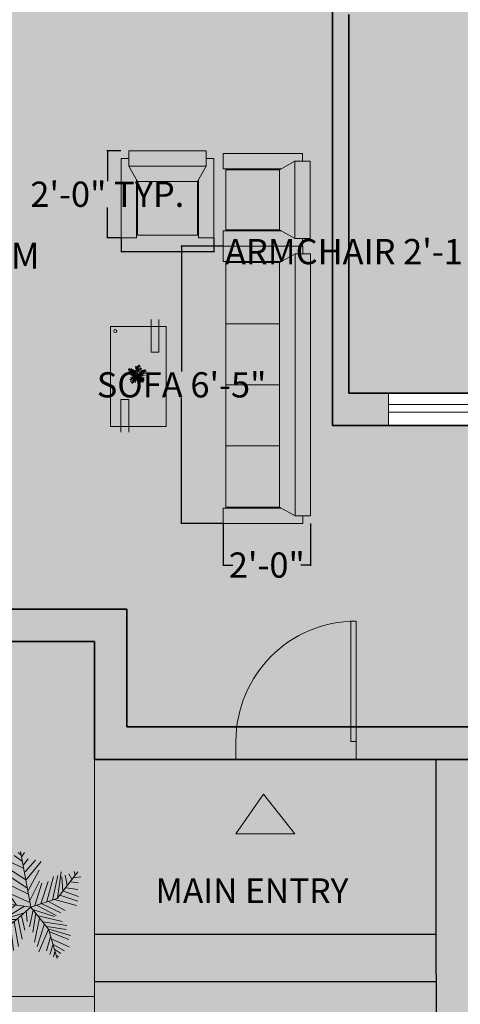
# Model space of a CAD drawing. Units: inches. Extents: x 1316 to 1777, y 813 to 1650.
# Tile 3 of 22: x 1481 to 1603, y 963 to 1237. Entities that reach past the tile are written whole.
import ezdxf

# ---------------------------------------------------------------- set-up
doc = ezdxf.new("R2010")
doc.units = ezdxf.units.IN
doc.header["$MEASUREMENT"] = 0
for name, color, linetype, lineweight in [('A-ANNO-DIMS', 2, 'Continuous', 18), ('A-ANNO-SYMB', 7, 'Continuous', 18), ('A-ANNO-SYMB-PATT', 7, 'Continuous', 13), ('A-AREA-IDEN', 7, 'Continuous', 18), ('A-DOOR', 4, 'Continuous', 18), ('A-DOOR-PATT', 253, 'Continuous', 13), ('A-FLOR-STRS', 7, 'Continuous', 25), ('A-FLOR-STRS-PATT', 252, 'Continuous', 13), ('A-FURN-PATT', 23, 'Continuous', 13), ('A-WALL-PATT', 250, 'Continuous', 13), ('furniture', 23, 'Continuous', 18), ('greenary', 106, 'Continuous', 13), ('L-HRDS', 8, 'Continuous', 18), ('L-HRDS-PATT', 252, 'Continuous', 13), ('L-PLNT-PATT', 74, 'Continuous', 13), ('text', 7, 'Continuous', 18), ('walls', 250, 'Continuous', 35), ('windows', 141, 'Continuous', 18)]:
    doc.layers.add(name, color=color, linetype=linetype, lineweight=lineweight)
doc.layers.add('A-FLOR-PATT', color=254, linetype='Continuous', lineweight=13, true_color=0xfeeab9)
doc.styles.get("Standard").update_dxf_attribs({"font": 'arial.ttf'})
doc.dimstyles.get("Standard").update_dxf_attribs({"dimtxt": 7, "dimasz": 0.18, "dimexe": 0.18, "dimexo": 0.0625, "dimgap": 0.09, "dimtad": 0, "dimtih": 1, "dimtoh": 1, "dimzin": 0, "dimdsep": 46, "dimlunit": 3, "dimtxsty": 'Standard', "dimcen": 0.09, "dimadec": 0, "dimazin": 0, "dimtfac": 1, "dimtofl": 0, "dimtmove": 0, "dimatfit": 3, "dimfxl": 1, "dimtolj": 1, "dimtzin": 0, "dimarcsym": 0})

# ---------------------------------------------------------------- blocks, each defined once
blk = doc.blocks.new('*U15')
for p, q in [((0, 0), (0, -6)), ((40, 0), (40, -6))]:
    blk.add_line(p, q)
blk.add_lwpolyline([(0, 0), (0, 40), (1.75, 40), (1.75, 0)], close=True)
blk.add_arc((0, 0), 40, 0, 90)
blk = doc.blocks.new('FABRIC SOFA 4S')
at = {"layer": 'furniture'}
for p, q in [((3, 54), (34, 54)), ((3, 51), (3, 54)), ((34, 48), (34, 54)), ((0, -51), (0, 51)), ((6, 51), (0, 51)), ((6, -51), (6, 51)), ((12, 47.63), (6, 51)), ((11.14, 48), (34, 48)), ((33, 23.81), (12, 23.81)), ((33, 0), (12, 0)), ((33, -23.81), (12, -23.81)), ((6, -51), (12, -47.63)), ((11.54, -48), (34, -48)), ((34, -48), (34, -54)), ((6, -51), (0, -51)), ((3, -54), (3, -51)), ((3, -54), (34, -54))]:
    blk.add_line(p, q, dxfattribs=at)
blk.add_lwpolyline([(12, -47.63), (12, 47.63), (33, 47.63), (33, -47.63)], close=True, dxfattribs=at)
blk = doc.blocks.new('*U13')
for p, q in [((-8.737, 47.138), (-17.069, 52.711)), ((-10.186, 53.64), (-13.084, 55.962)), ((0, 0), (-10.5, 57)), ((-9.099, 51.782), (-6.563, 55.962)), ((-5.114, 28.097), (-24.676, 40.636)), ((-7.288, 39.707), (-21.778, 46.673)), ((-7.65, 43.423), (-2.578, 49.46)), ((-5.839, 35.992), (4.667, 48.067)), ((-5.114, 27.632), (10.463, 46.673)), ((-3.665, 19.273), (-27.574, 35.527)), ((-2.941, 16.486), (8.652, 37.85)), ((16.259, 5.805), (23.142, 31.348)), ((22.055, 7.198), (27.489, 32.277)), ((27, 9), (48, 36)), ((27.127, 9.056), (31.112, 35.992)), ((31.836, 30.883), (32.561, 16.486)), ((35.096, 32.741), (37.27, 22.524)), ((38.719, 34.134), (41.979, 28.561)), ((43.791, 29.954), (51.036, 30.883)), ((44.153, 36.456), (45.239, 32.741)), ((-31.5, 4.5), (-52.5, 25.5)), ((-48.585, 21.131), (-49.309, 29.026)), ((-43.513, 28.561), (-42.427, 15.558)), ((-38.442, 26.239), (-34.819, 7.663)), ((-35.544, 28.097), (-24.314, 3.947)), ((-14.533, 2.09), (-30.834, 25.31)), ((-24.314, 23.917), (-2.941, 13.7)), ((-1.129, 6.734), (9.014, 26.704)), ((3.942, 1.625), (11.187, 24.381)), ((10.101, 3.483), (17.708, 26.239)), ((40.53, 25.775), (48.862, 24.846)), ((-47.498, 19.737), (-55.83, 18.344)), ((-40.615, 13.7), (-55.105, 10.913)), ((-20.691, 13.7), (-1.129, 4.876)), ((29.662, 12.307), (48.137, 6.269)), ((33.285, 16.486), (48.862, 10.913)), ((36.183, 19.737), (48.137, 17.88)), ((-33.37, 6.269), (-52.207, 5.34)), ((-28.299, 3.483), (-47.86, -5.805)), ((-21.416, 3.018), (-38.079, -8.128)), ((0, 0), (-31.5, 4.5)), ((-15.982, 2.09), (-30.11, -9.521)), ((0, 0), (-22.5, -19.5)), ((-6.563, 1.161), (-21.416, -8.128)), ((0, 0), (27, 9)), ((0, 0), (18, -22.5)), ((6.478, 1.625), (26.04, -8.592)), ((11.187, 3.483), (30.749, -5.805)), ((18.07, 5.805), (35.096, -3.483)), ((24.229, 7.663), (46.688, 1.625)), ((-6.563, -5.805), (-19.967, -9.985)), ((-9.461, -8.592), (-6.201, -23.453)), ((-4.752, -3.483), (-3.665, -14.629)), ((2.493, -3.019), (-1.491, -20.202)), ((1.769, -2.555), (24.229, -9.521)), ((5.029, -6.27), (2.131, -25.775)), ((7.565, -9.056), (32.198, -14.629)), ((-17.431, -15.094), (-42.789, -18.809)), ((-22.5, -19.5), (-37.5, -45)), ((-15.257, -12.772), (-30.11, -12.772)), ((-20.691, -18.345), (-17.793, -44.352)), ((-17.069, -15.094), (-12.721, -40.172)), ((-13.446, -11.378), (-8.737, -32.741)), ((9.014, -11.378), (3.58, -35.992)), ((14.085, -16.951), (6.478, -40.172)), ((12.274, -15.094), (36.907, -18.809)), ((16.259, -19.738), (36.183, -22.989)), ((-28.299, -29.026), (-42.789, -31.348)), ((-24.314, -21.596), (-42.427, -22.06)), ((-26.849, -26.24), (-40.253, -25.775)), ((-25.038, -23.918), (-22.865, -45.281)), ((18.07, -22.524), (8.289, -45.745)), ((18, -22.5), (27, -52.5)), ((18.433, -22.524), (40.53, -29.026)), ((19.157, -25.311), (38.719, -33.206)), ((-30.834, -34.135), (-42.427, -35.528)), ((-34.457, -39.708), (-40.978, -42.494)), ((-32.646, -36.921), (-31.921, -44.352)), ((-29.023, -30.884), (-27.936, -43.887)), ((20.244, -30.419), (15.897, -44.816)), ((22.78, -37.85), (19.519, -48.532)), ((21.331, -32.741), (39.081, -40.636)), ((22.78, -38.314), (34.372, -44.816)), ((24.591, -45.745), (23.142, -50.854)), ((24.591, -43.423), (30.749, -47.603)), ((26.764, -49.925), (28.213, -50.854))]:
    blk.add_line(p, q)
blk = doc.blocks.new('FABRIC SOFA 1S')
at = {"layer": 'furniture'}
for p, q in [((3, 18.12), (34, 18.12)), ((3, 15.12), (3, 18.12)), ((34, 12.12), (34, 18.12)), ((0, -15.12), (0, 15.12)), ((6, 15.12), (0, 15.12)), ((6, -15.12), (6, 15.12)), ((12, 11.75), (6, 15.12)), ((11.33, 12.12), (34, 12.12)), ((6, -15.12), (0, -15.12)), ((3, -18.12), (3, -15.12)), ((6, -15.12), (12, -11.75)), ((11.33, -12.12), (34, -12.12)), ((34, -12.12), (34, -18.12)), ((3, -18.12), (34, -18.12))]:
    blk.add_line(p, q, dxfattribs=at)
blk.add_lwpolyline([(12, -11.75), (12, 11.75), (33, 11.75), (33, -11.75)], close=True, dxfattribs=at)
blk = doc.blocks.new('*D32')
at = {"layer": 'A-ANNO-DIMS', "color": 0, "lineweight": -2, "transparency": 16777216}
for p, q in [((1508.99, 1175.95), (1508.99, 1171.97)), ((1534.72, 1175.95), (1534.72, 1171.97)), ((1509.17, 1172.15), (1534.54, 1172.15)), ((1534.72, 1172.15), (1534.9, 1172.15))]:
    blk.add_line(p, q, dxfattribs=at)
at = {"layer": 'A-ANNO-DIMS', "color": 0, "transparency": 16777216}
for points in [[(1509.17, 1172.18), (1509.17, 1172.12), (1508.99, 1172.15)], [(1534.54, 1172.18), (1534.54, 1172.12), (1534.72, 1172.15)]]:
    blk.add_solid(points, dxfattribs=at)
at = {"layer": 'Defpoints', "color": 0, "transparency": 16777216}
for p in [(1508.99, 1176.01), (1534.72, 1176.01), (1534.72, 1172.15)]:
    blk.add_point(p, dxfattribs=at)
at = {"layer": 'A-ANNO-DIMS', "color": 0, "transparency": 16777216, "insert": (1592.12, 1172.15), "char_height": 7, "attachment_point": 5}
blk.add_mtext('\\A1;ARMCHAIR 2\'-1 1/2" TYP.', dxfattribs=at)
blk = doc.blocks.new('*D33')
at = {"layer": 'A-ANNO-DIMS', "color": 0, "lineweight": -2, "transparency": 16777216}
for p, q in [((1508.92, 1200.15), (1504.95, 1200.15)), ((1505.13, 1199.97), (1505.13, 1191.74)), ((1505.13, 1176.19), (1505.13, 1184.41)), ((1508.92, 1176.01), (1504.95, 1176.01))]:
    blk.add_line(p, q, dxfattribs=at)
at = {"layer": 'A-ANNO-DIMS', "color": 0, "transparency": 16777216}
for points in [[(1505.1, 1199.97), (1505.16, 1199.97), (1505.13, 1200.15)], [(1505.1, 1176.19), (1505.16, 1176.19), (1505.13, 1176.01)]]:
    blk.add_solid(points, dxfattribs=at)
at = {"layer": 'Defpoints', "color": 0, "transparency": 16777216}
for p in [(1508.99, 1200.15), (1505.13, 1176.01), (1508.99, 1176.01)]:
    blk.add_point(p, dxfattribs=at)
at = {"layer": 'A-ANNO-DIMS', "color": 0, "transparency": 16777216, "insert": (1505.13, 1188.08), "char_height": 7, "attachment_point": 5}
blk.add_mtext('\\A1;2\'-0" TYP.', dxfattribs=at)
blk = doc.blocks.new('*D44')
at = {"layer": 'A-ANNO-DIMS', "color": 0, "lineweight": -2, "transparency": 16777216}
for p, q in [((1537.22, 1173.65), (1525.56, 1173.65)), ((1525.74, 1173.47), (1525.74, 1138.88)), ((1525.74, 1096.86), (1525.74, 1131.45)), ((1537.22, 1096.68), (1525.56, 1096.68))]:
    blk.add_line(p, q, dxfattribs=at)
at = {"layer": 'A-ANNO-DIMS', "color": 0, "transparency": 16777216}
for points in [[(1525.71, 1173.47), (1525.77, 1173.47), (1525.74, 1173.65)], [(1525.71, 1096.86), (1525.77, 1096.86), (1525.74, 1096.68)]]:
    blk.add_solid(points, dxfattribs=at)
at = {"layer": 'Defpoints', "color": 0, "transparency": 16777216}
for p in [(1525.74, 1173.65), (1537.28, 1173.65), (1537.28, 1096.68)]:
    blk.add_point(p, dxfattribs=at)
at = {"layer": 'A-ANNO-DIMS', "color": 0, "transparency": 16777216, "insert": (1525.74, 1135.17), "char_height": 7, "attachment_point": 5}
blk.add_mtext('\\A1;SOFA 6\'-5"', dxfattribs=at)
blk = doc.blocks.new('*D45')
at = {"layer": 'A-ANNO-DIMS', "color": 0, "lineweight": -2, "transparency": 16777216}
for p, q in [((1537.28, 1096.62), (1537.28, 1084.95)), ((1561.52, 1096.62), (1561.52, 1084.95)), ((1537.46, 1085.13), (1539.95, 1085.13)), ((1561.34, 1085.13), (1558.85, 1085.13))]:
    blk.add_line(p, q, dxfattribs=at)
at = {"layer": 'A-ANNO-DIMS', "color": 0, "transparency": 16777216}
for points in [[(1537.46, 1085.16), (1537.46, 1085.1), (1537.28, 1085.13)], [(1561.34, 1085.16), (1561.34, 1085.1), (1561.52, 1085.13)]]:
    blk.add_solid(points, dxfattribs=at)
at = {"layer": 'Defpoints', "color": 0, "transparency": 16777216}
for p in [(1537.28, 1096.68), (1561.52, 1096.68), (1537.28, 1085.13)]:
    blk.add_point(p, dxfattribs=at)
at = {"layer": 'A-ANNO-DIMS', "color": 0, "transparency": 16777216, "insert": (1549.4, 1085.13), "char_height": 7, "attachment_point": 5}
blk.add_mtext('\\A1;2\'-0"', dxfattribs=at)
blk = doc.blocks.new('*D50')
at = {"layer": 'A-ANNO-DIMS', "color": 0, "lineweight": -2, "transparency": 16777216}
for p, q in [((1377.06, 1063.81), (1377.06, 817.77)), ((1713.17, 1031.11), (1713.17, 817.77)), ((1377.24, 817.95), (1532.95, 817.95)), ((1712.99, 817.95), (1557.29, 817.95))]:
    blk.add_line(p, q, dxfattribs=at)
at = {"layer": 'A-ANNO-DIMS', "color": 0, "transparency": 16777216}
for points in [[(1377.24, 817.98), (1377.24, 817.92), (1377.06, 817.95)], [(1712.99, 817.98), (1712.99, 817.92), (1713.17, 817.95)]]:
    blk.add_solid(points, dxfattribs=at)
at = {"layer": 'Defpoints', "color": 0, "transparency": 16777216}
for p in [(1377.06, 1063.87), (1713.17, 1031.17), (1713.17, 817.95)]:
    blk.add_point(p, dxfattribs=at)
at = {"layer": 'A-ANNO-DIMS', "color": 0, "transparency": 16777216, "insert": (1545.12, 817.95), "char_height": 7, "attachment_point": 5}
blk.add_mtext('\\A1;28\'-0"', dxfattribs=at)

msp = doc.modelspace()

# ---------------------------------------------------------------- hatches: boundary and pattern name
at = {"layer": 'A-ANNO-SYMB-PATT'}
h = msp.add_hatch(color=256, dxfattribs=at)
h.dxf.hatch_style = 1
h.paths.add_polyline_path([(1548.475, 1021.524), (1540.783, 1010.496), (1557.193, 1010.496)])
at = {"layer": 'A-DOOR-PATT'}
h = msp.add_hatch(color=256, dxfattribs=at)
h.dxf.hatch_style = 1
h.paths.add_polyline_path([(1601.07, 1266.995), (1572.173, 1266.995), (1572.173, 1265.725), (1601.042, 1265.725, 0.0109414)])
h.paths.add_polyline_path([(1574.225, 1069.579, 0.0109414), (1572.764, 1069.547), (1572.764, 1040.173), (1574.225, 1040.173)])
h.paths.add_polyline_path([(1574.225, 1040.173), (1572.764, 1040.173), (1572.764, 1036.182), (1574.225, 1036.182)])
at = {"layer": 'A-FLOR-PATT'}
h = msp.add_hatch(color=256, dxfattribs=at)
h.dxf.hatch_style = 1
h.paths.add_polyline_path([(1567.673, 1281.369), (1651.673, 1281.369), (1651.673, 1365.369), (1597.673, 1365.369), (1597.673, 1429.869), (1570.345, 1429.869), (1570.345, 1471.869), (1510.345, 1471.869), (1510.345, 1429.869), (1444.564, 1429.869), (1444.564, 1322.882), (1444.564, 1300.088), (1510.564, 1300.088), (1510.564, 1295.094), (1510.564, 1240.869), (1386.064, 1240.869), (1386.064, 1171.185), (1400.961, 1171.185), (1400.961, 1106.742), (1386.064, 1106.742), (1386.064, 1072.869), (1510.564, 1072.869), (1510.564, 1040.173), (1541.068, 1040.173, -0.367085), (1572.764, 1069.547), (1572.764, 1069.579), (1574.225, 1069.579), (1574.225, 1040.173), (1616.037, 1040.173), (1616.037, 1086.627), (1616.037, 1103.705), (1613.066, 1105.235), (1616.037, 1106.686), (1616.037, 1123.869), (1567.673, 1123.869)])
h.paths.add_polyline_path([(1508.987, 1198.018), (1511.117, 1198.018), (1511.117, 1200.148), (1532.595, 1200.148), (1532.595, 1198.018), (1534.725, 1198.018), (1534.725, 1176.008), (1530.465, 1176.008), (1530.465, 1176.718), (1513.247, 1176.718), (1513.247, 1176.008), (1508.987, 1176.008)], flags=16)
h.paths.add_polyline_path([(1505.979, 1151.315), (1521.504, 1151.315), (1521.504, 1123.623), (1505.979, 1123.623)], flags=16)
h.paths.add_polyline_path([(1507.734, 1150.101, -1), (1506.932, 1150.101, -1)], flags=0)
h.paths.add_polyline_path([(1512.288, 1138.353), (1512.28, 1138.392), (1512.219, 1138.376)], flags=0)
h.paths.add_polyline_path([(1511.539, 1138.926), (1511.802, 1138.967), (1511.817, 1139.27), (1511.607, 1139.246)], flags=0)
h.paths.add_polyline_path([(1513.745, 1140.234), (1513.68, 1139.885), (1514.014, 1140.045), (1513.855, 1140.308)], flags=0)
h.paths.add_polyline_path([(1513.759, 1139.089), (1514.005, 1139.255), (1513.807, 1139.483), (1513.564, 1139.327)], flags=0)
h.paths.add_polyline_path([(1514.219, 1138.385), (1514.336, 1138.33), (1514.544, 1138.32), (1514.802, 1138.874), (1514.451, 1138.716)], flags=0)
h.paths.add_polyline_path([(1514.577, 1137.439), (1514.573, 1137.4), (1514.699, 1137.4), (1514.696, 1137.402)], flags=0)
h.paths.add_polyline_path([(1512.26, 1136.199), (1512.199, 1136.399), (1512.032, 1136.325), (1512.095, 1136.101), (1512.257, 1136.192)], flags=0)
h.paths.add_polyline_path([(1512.644, 1137.274), (1512.356, 1137.23), (1512.432, 1137.049), (1512.703, 1137.093)], flags=0)
h.paths.add_polyline_path([(1513.049, 1137.593), (1512.979, 1137.8), (1512.843, 1137.757), (1512.887, 1137.556)], flags=0)
h.paths.add_polyline_path([(1513.269, 1138.556), (1513.571, 1137.962), (1513.459, 1136.814), (1513.212, 1137.878), (1513.032, 1138.443)], flags=0)
h.paths.add_polyline_path([(1514.891, 1136.377), (1514.696, 1136.401), (1514.683, 1136.246), (1514.87, 1136.165)], flags=0)
h.paths.add_polyline_path([(1514.142, 1137.293), (1514.047, 1136.743), (1514.27, 1136.751), (1514.328, 1137.265)], flags=0)
h.paths.add_polyline_path([(1515.362, 1138.976), (1515.334, 1138.638), (1515.596, 1138.588), (1515.627, 1138.932)], flags=0)
h.paths.add_polyline_path([(1537.285, 1177.912), (1537.995, 1177.912), (1537.995, 1195.13), (1537.285, 1195.13), (1537.285, 1199.39), (1559.295, 1199.39), (1559.295, 1197.26), (1561.425, 1197.26), (1561.425, 1175.782), (1559.295, 1175.782), (1559.295, 1173.652), (1559.379, 1173.652), (1559.379, 1171.514), (1561.517, 1171.514), (1561.517, 1098.819), (1559.379, 1098.819), (1559.379, 1096.68), (1537.285, 1096.68), (1537.285, 1100.957), (1537.997, 1100.957), (1537.997, 1169.376), (1537.285, 1169.376), (1537.285, 1173.652)], flags=16)
h.paths.add_polyline_path([(1518.623, 1345.565), (1519.133, 1345.48), (1519.133, 1345.485), (1518.623, 1345.567)], flags=16)
h.paths.add_polyline_path([(1518.798, 1374.15), (1519.308, 1374.064), (1519.308, 1374.069), (1518.798, 1374.152)], flags=16)
h.paths.add_polyline_path([(1537.764, 1413.501), (1537.678, 1412.991), (1537.683, 1412.991), (1537.766, 1413.501)], flags=16)
h.paths.add_polyline_path([(1572.905, 1373.821), (1573.927, 1373.975), (1574.027, 1390.309), (1573.007, 1390.475), (1573.007, 1390.475)], flags=16)
h.paths.add_polyline_path([(1572.73, 1345.237), (1573.752, 1345.39), (1573.852, 1361.724), (1572.832, 1361.89), (1572.832, 1361.89)], flags=16)
h.paths.add_polyline_path([(1537.211, 1322.643), (1537.364, 1321.621), (1553.698, 1321.521), (1553.864, 1322.541)], flags=16)
h.paths.add_polyline_path([(1535.908, 1331.328), (1527.214, 1331.382), (1527.664, 1404.885), (1564.416, 1404.66), (1563.966, 1331.157), (1555.273, 1331.21), (1553.947, 1323.051), (1537.134, 1323.154)], flags=16)
h.paths.add_polyline_path([(1536.15, 1336.503), (1536.235, 1337.572), (1536.323, 1338.628), (1536.411, 1339.663), (1536.495, 1340.67), (1536.574, 1341.66), (1536.648, 1342.648), (1536.717, 1343.649), (1536.78, 1344.678), (1536.837, 1345.75), (1536.913, 1347.475), (1536.93, 1348.082), (1536.867, 1346.314), (1536.754, 1344.188), (1536.619, 1342.219), (1536.495, 1340.67), (1536.411, 1339.663), (1536.323, 1338.628), (1536.235, 1337.572), (1536.15, 1336.503), (1536.071, 1335.432), (1536.002, 1334.37), (1535.917, 1332.754), (1535.909, 1332.308), (1535.964, 1333.78), (1536.071, 1335.432)], flags=0)
h.paths.add_polyline_path([(1540.412, 1338.345), (1540.539, 1339.037), (1540.667, 1339.758), (1540.798, 1340.518), (1540.93, 1341.325), (1541.063, 1342.187), (1541.196, 1343.109), (1541.326, 1344.085), (1541.45, 1345.102), (1541.566, 1346.15), (1541.669, 1347.219), (1541.758, 1348.296), (1541.829, 1349.371), (1541.879, 1350.434), (1541.906, 1351.476), (1541.91, 1352.5), (1541.895, 1353.512), (1541.861, 1354.518), (1541.812, 1355.524), (1541.749, 1356.537), (1541.674, 1357.561), (1541.551, 1359.062), (1541.495, 1359.67), (1541.589, 1358.603), (1541.721, 1356.977), (1541.846, 1354.98), (1541.912, 1352.982), (1541.903, 1350.951), (1541.806, 1348.87), (1541.628, 1346.713), (1541.396, 1344.612), (1541.135, 1342.656), (1540.872, 1340.947), (1540.617, 1339.466), (1540.412, 1338.345), (1540.288, 1337.675), (1540.166, 1337.018), (1540.049, 1336.365), (1539.937, 1335.71), (1539.837, 1335.055), (1539.758, 1334.403), (1539.709, 1333.756), (1539.697, 1333.12), (1539.751, 1332.162), (1539.822, 1331.89), (1539.691, 1332.775), (1539.714, 1334.035), (1539.867, 1335.303), (1540.085, 1336.577), (1540.288, 1337.675)], flags=0)
h.paths.add_polyline_path([(1545.599, 1331.584), (1545.601, 1331.617), (1545.614, 1331.689), (1545.737, 1332.197), (1545.767, 1332.332), (1545.84, 1332.681), (1545.925, 1333.114), (1546.016, 1333.614), (1546.108, 1334.164), (1546.196, 1334.748), (1546.276, 1335.349), (1546.342, 1335.952), (1546.388, 1336.539), (1546.412, 1337.098), (1546.414, 1337.632), (1546.395, 1338.145), (1546.359, 1338.645), (1546.306, 1339.137), (1546.24, 1339.627), (1546.161, 1340.121), (1546.073, 1340.625), (1545.888, 1341.63), (1545.718, 1342.621), (1545.547, 1343.945), (1545.432, 1345.534), (1545.404, 1347.402), (1545.418, 1348.013), (1545.411, 1346.957), (1545.425, 1345.988), (1545.463, 1345.105), (1545.521, 1344.301), (1545.596, 1343.566), (1545.683, 1342.892), (1545.778, 1342.27), (1545.877, 1341.691), (1545.977, 1341.145), (1546.133, 1340.297), (1546.327, 1339.075), (1546.434, 1337.615), (1546.377, 1336.279), (1546.246, 1335.079), (1546.032, 1333.665), (1545.84, 1332.681), (1545.767, 1332.332)], flags=0)
h.paths.add_polyline_path([(1551.803, 1337.656), (1551.963, 1338.25), (1552.102, 1338.801), (1552.225, 1339.338), (1552.331, 1339.865), (1552.418, 1340.377), (1552.487, 1340.873), (1552.536, 1341.348), (1552.563, 1341.801), (1552.569, 1342.228), (1552.551, 1342.627), (1552.51, 1342.995), (1552.446, 1343.333), (1552.363, 1343.646), (1552.261, 1343.937), (1552.144, 1344.207), (1552.012, 1344.461), (1551.868, 1344.7), (1551.746, 1344.882), (1550.887, 1346.052), (1550.428, 1347.126), (1550.183, 1348.353), (1550.048, 1349.632), (1549.978, 1351.224), (1549.974, 1353.141), (1549.989, 1353.748), (1549.975, 1352.682), (1549.977, 1351.708), (1549.996, 1350.825), (1550.031, 1350.027), (1550.082, 1349.31), (1550.15, 1348.669), (1550.234, 1348.098), (1550.335, 1347.593), (1550.452, 1347.149), (1550.584, 1346.76), (1550.73, 1346.419), (1550.887, 1346.117), (1551.05, 1345.848), (1551.217, 1345.602), (1551.386, 1345.372), (1551.553, 1345.151), (1552, 1344.537), (1552.454, 1343.495), (1552.591, 1342.266), (1552.509, 1340.905), (1552.246, 1339.367), (1551.925, 1338.101), (1551.619, 1336.984), (1551.406, 1336.2), (1551.01, 1334.699), (1550.877, 1334.155), (1551.264, 1335.677), (1551.619, 1336.984)], flags=0)
h.paths.add_polyline_path([(1558.642, 1348.348), (1558.795, 1348.811), (1558.918, 1349.215), (1559.008, 1349.575), (1559.061, 1349.904), (1559.076, 1350.214), (1559.054, 1350.506), (1559.001, 1350.776), (1558.919, 1351.021), (1558.814, 1351.239), (1558.688, 1351.425), (1558.546, 1351.578), (1558.392, 1351.694), (1558.229, 1351.772), (1558.059, 1351.812), (1557.882, 1351.819), (1557.701, 1351.794), (1557.515, 1351.742), (1557.327, 1351.665), (1557.136, 1351.566), (1556.944, 1351.448), (1556.752, 1351.315), (1556.742, 1351.307), (1556.175, 1350.878), (1555.982, 1350.741), (1555.79, 1350.618), (1555.103, 1350.248), (1554.019, 1350.696), (1553.658, 1351.734), (1553.592, 1352.861), (1553.705, 1354.248), (1553.753, 1354.657), (1553.685, 1354.004), (1553.638, 1353.425), (1553.615, 1352.918), (1553.615, 1352.476), (1553.637, 1352.094), (1553.681, 1351.766), (1553.745, 1351.485), (1553.828, 1351.246), (1553.929, 1351.043), (1554.048, 1350.87), (1554.182, 1350.722), (1554.33, 1350.599), (1554.491, 1350.501), (1554.662, 1350.43), (1554.841, 1350.388), (1555.026, 1350.374), (1555.215, 1350.39), (1555.406, 1350.437), (1555.598, 1350.514), (1555.79, 1350.618), (1555.982, 1350.741), (1556.175, 1350.878), (1556.367, 1351.024), (1556.559, 1351.171), (1556.752, 1351.315), (1556.944, 1351.448), (1557.136, 1351.566), (1557.327, 1351.665), (1558.043, 1351.957), (1558.894, 1351.316), (1559.137, 1350.09), (1558.886, 1349.087), (1558.642, 1348.348), (1558.463, 1347.812), (1558.261, 1347.187), (1558.039, 1346.459), (1557.677, 1345.175), (1557.549, 1344.636), (1557.909, 1346.03), (1558.329, 1347.408)], flags=0)
h.paths.add_polyline_path([(1562.145, 1353.919), (1562.25, 1354.68), (1562.341, 1355.344), (1562.416, 1355.924), (1562.475, 1356.431), (1562.518, 1356.872), (1562.544, 1357.254), (1562.554, 1357.582), (1562.548, 1357.862), (1562.525, 1358.1), (1562.486, 1358.303), (1562.432, 1358.476), (1562.361, 1358.624), (1562.277, 1358.748), (1562.18, 1358.848), (1562.073, 1358.925), (1561.958, 1358.977), (1561.837, 1359.006), (1561.711, 1359.011), (1561.584, 1358.992), (1561.456, 1358.949), (1561.342, 1358.895), (1560.78, 1358.554), (1560.631, 1358.473), (1560.474, 1358.403), (1560.311, 1358.348), (1559.637, 1358.207), (1558.973, 1358.904), (1558.816, 1360.002), (1558.804, 1361.236), (1558.83, 1361.674), (1558.807, 1360.917), (1558.813, 1360.297), (1558.845, 1359.795), (1558.902, 1359.397), (1558.982, 1359.087), (1559.082, 1358.849), (1559.2, 1358.666), (1559.334, 1358.525), (1559.482, 1358.421), (1559.639, 1358.351), (1559.804, 1358.311), (1559.973, 1358.3), (1560.143, 1358.313), (1560.311, 1358.348), (1560.474, 1358.403), (1560.631, 1358.473), (1560.78, 1358.554), (1560.923, 1358.641), (1561.061, 1358.729), (1561.196, 1358.813), (1561.382, 1358.92), (1561.342, 1358.895), (1561.972, 1359.194), (1562.536, 1358.367), (1562.56, 1357.311), (1562.455, 1356.226), (1562.323, 1355.206), (1562.145, 1353.919), (1562.026, 1353.049), (1561.815, 1351.457), (1561.752, 1350.933), (1561.948, 1352.479)], flags=0)
h.paths.add_polyline_path([(1572.764, 1069.547, 0.367085), (1541.068, 1040.173), (1572.764, 1040.173)], flags=17)
h.paths.add_polyline_path([(1572.764, 1040.173), (1541.068, 1040.173, 0.0299535), (1540.829, 1036.182), (1540.829, 1031.173), (1574.225, 1031.173), (1574.225, 1036.182), (1572.764, 1036.182)])
h = msp.add_hatch(color=256, dxfattribs=at)
h.dxf.hatch_style = 1
h.paths.add_polyline_path([(1704.173, 1260.711), (1625.405, 1260.711), (1625.405, 1261.154), (1625.405, 1276.279), (1624.85, 1276.279), (1572.173, 1276.869), (1572.173, 1266.995), (1601.07, 1266.995), (1601.07, 1265.725), (1601.042, 1265.725, -0.4000145), (1572.173, 1237.955), (1572.173, 1132.869), (1704.173, 1132.869)])
edge = h.paths.add_edge_path(flags=0)
edge.add_spline(control_points=[(1634.063, 1215.447), (1634.008, 1215.524), (1633.887, 1215.694), (1634.084, 1216.011), (1634.356, 1216.402), (1634.084, 1216.621), (1633.946, 1216.732)], knot_values=[0, 0, 0, 0, 0.3739943, 0.8243137, 1.461173, 2.1144513, 2.1144513, 2.1144513, 2.1144513], degree=3, periodic=0)
edge.add_spline(control_points=[(1633.711, 1215.447), (1633.656, 1215.524), (1633.535, 1215.694), (1633.732, 1216.011), (1634.005, 1216.402), (1633.732, 1216.621), (1633.594, 1216.732)], knot_values=[0, 0, 0, 0, 0.3739943, 0.8243137, 1.461173, 2.1144513, 2.1144513, 2.1144513, 2.1144513], degree=3, periodic=0)
edge = h.paths.add_edge_path(flags=16)
edge.add_line((1631.459, 1215.447), (1661.482, 1215.447))
edge.add_line((1661.482, 1215.447), (1661.482, 1208.307))
edge.add_line((1661.482, 1208.307), (1688.953, 1208.307))
edge.add_line((1688.953, 1208.307), (1688.837, 1220.405))
edge.add_line((1688.837, 1220.405), (1702.711, 1220.405))
edge.add_line((1702.711, 1220.405), (1702.827, 1208.307))
edge.add_line((1702.827, 1208.307), (1702.827, 1154.307))
edge.add_line((1702.827, 1154.307), (1702.944, 1142.208))
edge.add_line((1702.944, 1142.208), (1689.07, 1142.208))
edge.add_line((1689.07, 1142.208), (1688.953, 1154.307))
edge.add_line((1688.953, 1154.307), (1661.482, 1154.307))
edge.add_line((1661.482, 1154.307), (1661.482, 1143.444))
edge.add_line((1661.482, 1143.444), (1634.022, 1143.444))
edge.add_spline(control_points=[(1634.022, 1143.444), (1633.972, 1143.371), (1633.857, 1143.204), (1634.053, 1142.892), (1634.324, 1142.501), (1634.052, 1142.282), (1633.914, 1142.172)], knot_values=[0, 0, 0, 0, 0.3521435, 0.8024629, 1.4393222, 2.0926005, 2.0926005, 2.0926005, 2.0926005], degree=3, periodic=0)
edge.add_spline(control_points=[(1633.562, 1142.172), (1633.7, 1142.282), (1633.973, 1142.501), (1633.701, 1142.892), (1633.505, 1143.204), (1633.62, 1143.371), (1633.67, 1143.444)], knot_values=[0, 0, 0, 0, 0.6532783, 1.2901376, 1.740457, 2.0926005, 2.0926005, 2.0926005, 2.0926005], degree=3, periodic=0)
edge.add_line((1633.67, 1143.444), (1631.459, 1143.444))
edge.add_line((1631.459, 1143.444), (1631.459, 1215.447))
h.paths.add_polyline_path([(1691.549, 1164.108), (1691.597, 1164.173), (1691.597, 1202.209), (1699.757, 1202.209), (1699.757, 1186.386), (1691.597, 1186.386), (1691.597, 1179.931), (1699.757, 1179.931), (1699.757, 1164.108), (1691.549, 1164.108), (1684.365, 1154.365), (1684.365, 1164.108)], flags=0)
h.paths.add_polyline_path([(1691.424, 1214.03, -1), (1700.356, 1214.03, -1)], flags=0)
h.paths.add_polyline_path([(1691.541, 1147.932, -1), (1700.473, 1147.932, -1)], flags=0)
h.paths.add_polyline_path([(1601.042, 1265.725), (1572.029, 1265.725), (1572.029, 1266.995), (1567.673, 1266.995), (1567.673, 1237.955), (1572.029, 1237.955, 0.4014527)])
at = {"layer": 'A-FLOR-STRS-PATT'}
h = msp.add_hatch(color=256, dxfattribs=at)
h.dxf.hatch_style = 1
h.paths.add_polyline_path([(1596.428, 1031.173), (1501.564, 1031.173), (1501.564, 982.68), (1596.428, 982.68)])
h = msp.add_hatch(color=256, dxfattribs=at)
h.dxf.hatch_style = 1
h.paths.add_polyline_path([(1596.428, 982.68), (1501.564, 982.68), (1501.564, 969.464), (1596.428, 969.464), (1596.428, 971.474)])
h.paths.add_polyline_path([(1596.428, 969.464), (1501.564, 969.464), (1501.564, 965.355), (1501.564, 953.689), (1551.506, 953.689), (1551.506, 955.706), (1553.55, 955.706), (1553.55, 953.689), (1596.428, 953.689)])
at = {"layer": 'A-FURN-PATT'}
h = msp.add_hatch(color=256, dxfattribs=at)
h.dxf.hatch_style = 1
h.paths.add_polyline_path([(1530.199, 1191.628), (1513.514, 1191.628), (1513.514, 1176.718), (1530.199, 1176.718)])
h.paths.add_polyline_path([(1532.595, 1195.888), (1511.117, 1195.888), (1513.514, 1191.628), (1530.199, 1191.628)])
h.paths.add_polyline_path([(1532.595, 1200.148), (1511.117, 1200.148), (1511.117, 1195.888), (1532.595, 1195.888)])
h.paths.add_polyline_path([(1513.247, 1192.101), (1511.117, 1195.888), (1511.117, 1198.018), (1508.987, 1198.018), (1508.987, 1176.008), (1513.247, 1176.008)])
h.paths.add_polyline_path([(1534.725, 1198.018), (1532.595, 1198.018), (1532.595, 1195.888), (1530.465, 1192.101), (1530.465, 1176.008), (1534.725, 1176.008)])
h.paths.add_polyline_path([(1552.905, 1194.864), (1537.995, 1194.864), (1537.995, 1178.179), (1552.905, 1178.179)])
h.paths.add_polyline_path([(1557.165, 1197.26), (1559.295, 1197.26), (1559.295, 1199.39), (1537.285, 1199.39), (1537.285, 1195.13), (1553.378, 1195.13)])
h.paths.add_polyline_path([(1561.425, 1197.26), (1557.165, 1197.26), (1557.165, 1175.782), (1561.425, 1175.782)])
h.paths.add_polyline_path([(1557.165, 1197.26), (1552.905, 1194.864), (1552.905, 1178.179), (1557.165, 1175.782)])
h.paths.add_polyline_path([(1559.295, 1175.782), (1557.165, 1175.782), (1553.378, 1177.912), (1537.285, 1177.912), (1537.285, 1173.652), (1559.295, 1173.652)])
h.paths.add_polyline_path([(1559.379, 1173.652), (1537.285, 1173.652), (1537.285, 1169.376), (1553.439, 1169.376), (1557.241, 1171.514), (1559.379, 1171.514)])
h.paths.add_polyline_path([(1559.379, 1096.68), (1537.285, 1096.68), (1537.285, 1100.957), (1553.439, 1100.957), (1557.241, 1098.819), (1559.379, 1098.819)])
h.paths.add_polyline_path([(1552.964, 1118.195), (1537.997, 1118.195), (1537.997, 1101.224), (1552.964, 1101.224)])
h.paths.add_polyline_path([(1552.964, 1135.166), (1537.997, 1135.166), (1537.997, 1118.195), (1552.964, 1118.195)])
h.paths.add_polyline_path([(1552.964, 1152.138), (1537.997, 1152.138), (1537.997, 1135.166), (1552.964, 1135.166)])
h.paths.add_polyline_path([(1552.964, 1169.109), (1537.997, 1169.109), (1537.997, 1152.138), (1552.964, 1152.138)])
h.paths.add_polyline_path([(1557.241, 1171.514), (1552.964, 1169.109), (1552.964, 1101.224), (1557.241, 1098.819)])
h.paths.add_polyline_path([(1561.517, 1171.514), (1557.241, 1171.514), (1557.241, 1098.819), (1561.517, 1098.819)])
h = msp.add_hatch(color=256, dxfattribs=at)
h.dxf.hatch_style = 1
h.paths.add_polyline_path([(1505.979, 1151.315), (1517.273, 1151.315), (1517.273, 1144.19), (1519.467, 1144.19), (1519.467, 1151.315), (1521.504, 1151.315), (1521.504, 1123.623), (1511.114, 1123.623), (1511.114, 1131.093), (1508.921, 1131.093), (1508.921, 1123.623), (1505.979, 1123.623)])
h.paths.add_polyline_path([(1514.021, 1138.103), (1514.047, 1138.139), (1514.081, 1138.111)], flags=16)
h.paths.add_polyline_path([(1515.636, 1139.029), (1514.909, 1138.302), (1514.969, 1138.299), (1514.984, 1138.377), (1515.552, 1138.944), (1515.627, 1138.932)], flags=16)
h.paths.add_polyline_path([(1512.26, 1136.199), (1512.261, 1136.194), (1512.257, 1136.192)], flags=16)
h.paths.add_polyline_path([(1513.564, 1139.327), (1513.575, 1139.314), (1513.334, 1138.005), (1512.858, 1138.163), (1512.849, 1138.191), (1512.819, 1138.176), (1512.056, 1138.431), (1511.792, 1138.77), (1511.793, 1138.798), (1511.775, 1138.791), (1512.049, 1138.44), (1512.05, 1138.433), (1513.334, 1138.005), (1513.233, 1137.878), (1513.213, 1137.872), (1513.217, 1137.858), (1512.764, 1137.292), (1512.644, 1137.274), (1512.674, 1137.18), (1512.487, 1136.946), (1512.477, 1136.943), (1512.479, 1136.936), (1513.334, 1138.005), (1514.144, 1137.303), (1514.142, 1137.293), (1514.158, 1137.29), (1513.334, 1138.005), (1513.579, 1139.337)], flags=16)
h.paths.add_polyline_path([(1507.734, 1150.101, 1), (1506.932, 1150.101, 1)], flags=16)
h = msp.add_hatch(color=256, dxfattribs=at)
h.dxf.hatch_style = 1
h.paths.add_polyline_path([(1517.273, 1151.315), (1519.467, 1151.315), (1519.467, 1144.19), (1517.273, 1144.19)])
h.paths.add_polyline_path([(1517.273, 1153.28), (1519.467, 1153.28), (1519.467, 1151.315), (1517.273, 1151.315)])
h.paths.add_polyline_path([(1508.921, 1131.093), (1511.114, 1131.093), (1511.114, 1123.623), (1508.921, 1123.623)])
h.paths.add_polyline_path([(1508.921, 1123.623), (1511.114, 1123.623), (1511.114, 1122.002), (1508.921, 1122.002)])
at = {"layer": 'A-WALL-PATT'}
h = msp.add_hatch(color=256, dxfattribs=at)
h.dxf.hatch_style = 1
h.paths.add_polyline_path([(1713.173, 1281.369), (1656.173, 1281.369), (1656.173, 1298.258), (1651.673, 1298.258), (1651.673, 1281.369), (1567.673, 1281.369), (1567.673, 1266.995), (1572.173, 1266.995), (1572.173, 1276.869), (1704.173, 1276.869), (1704.173, 1132.869), (1608.64, 1132.869), (1608.64, 1123.869), (1704.173, 1123.869), (1704.173, 1040.173), (1652.869, 1040.173), (1652.869, 1031.173), (1713.173, 1031.173), (1713.173, 1040.173)])
h.paths.add_polyline_path([(1572.173, 1237.955), (1567.673, 1237.955), (1567.673, 1123.869), (1583.146, 1123.869), (1583.146, 1132.869), (1572.173, 1132.869)], flags=17)
h.paths.add_polyline_path([(1510.345, 1566.369), (1524.171, 1566.369), (1524.171, 1571.985), (1524.171, 1575.369), (1445.955, 1575.369), (1445.955, 1566.369), (1505.845, 1566.369), (1505.845, 1469.591), (1510.345, 1469.591), (1510.345, 1471.869), (1529.081, 1471.869), (1529.081, 1476.369), (1510.345, 1476.369)])
h.paths.add_polyline_path([(1609.722, 1575.369), (1545.119, 1575.369), (1545.119, 1566.369), (1570.345, 1566.369), (1570.345, 1476.369), (1562.477, 1476.369), (1562.477, 1471.869), (1570.345, 1471.869), (1570.345, 1469.591), (1574.845, 1469.591), (1574.845, 1566.369), (1609.722, 1566.369)])
h.paths.add_polyline_path([(1713.173, 1575.369), (1655.233, 1575.369), (1655.233, 1566.369), (1704.173, 1566.369), (1704.173, 1434.369), (1574.845, 1434.369), (1574.845, 1440.551), (1574.701, 1440.551), (1570.345, 1440.551), (1570.345, 1429.869), (1597.673, 1429.869), (1597.673, 1408.281), (1602.173, 1408.281), (1602.173, 1429.869), (1704.173, 1429.869), (1704.173, 1410.704), (1707.375, 1410.704), (1713.173, 1410.704)])
h.paths.add_polyline_path([(1713.173, 1383.676), (1704.173, 1383.676), (1704.173, 1369.869), (1602.173, 1369.869), (1602.173, 1379.241), (1597.673, 1379.241), (1597.673, 1365.369), (1713.173, 1365.369)])
h.paths.add_polyline_path([(1444.564, 1429.869), (1510.345, 1429.869), (1510.345, 1440.551), (1505.845, 1440.551), (1505.845, 1434.369), (1386.064, 1434.369), (1386.064, 1566.369), (1400.445, 1566.369), (1400.445, 1575.369), (1377.064, 1575.369), (1377.064, 1412.813), (1380.509, 1412.813), (1386.064, 1412.813), (1386.064, 1429.869), (1440.064, 1429.869), (1440.064, 1401.229), (1444.564, 1401.229)])
h.paths.add_polyline_path([(1444.564, 1372.189), (1440.064, 1372.189), (1440.064, 1369.869), (1386.064, 1369.869), (1386.064, 1378.758), (1377.064, 1378.758), (1377.064, 1349.201), (1381.118, 1349.201), (1386.064, 1349.201), (1386.064, 1365.369), (1440.064, 1365.369), (1440.064, 1322.882), (1444.564, 1322.882)])
h.paths.add_polyline_path([(1510.564, 1295.094), (1506.064, 1295.094), (1506.064, 1245.369), (1386.064, 1245.369), (1386.064, 1272.582), (1377.064, 1272.582), (1377.064, 1212.905), (1380.1, 1212.905), (1386.064, 1212.905), (1386.064, 1240.869), (1510.564, 1240.869)])
h.paths.add_polyline_path([(1386.064, 1163.761), (1377.064, 1163.761), (1377.064, 1063.869), (1419.363, 1063.869), (1419.363, 1072.869), (1386.064, 1072.869)])
h.paths.add_polyline_path([(1510.564, 1072.869), (1469.381, 1072.869), (1469.381, 1063.869), (1501.564, 1063.869), (1501.564, 1033.023), (1501.564, 1031.173), (1540.829, 1031.173), (1540.829, 1036.182, -0.0299535), (1541.068, 1040.173), (1510.564, 1040.173)])
h.paths.add_polyline_path([(1607.369, 1040.173), (1574.225, 1040.173), (1574.225, 1036.182), (1574.225, 1031.173), (1607.369, 1031.173)], flags=17)
h.paths.add_polyline_path([(1637.054, 1040.173), (1624.706, 1040.173), (1624.706, 1031.173), (1637.054, 1031.173)], flags=17)
at = {"layer": 'L-HRDS-PATT'}
h = msp.add_hatch(color=256, dxfattribs=at)
h.dxf.hatch_style = 1
h.paths.add_polyline_path([(1501.564, 965.355), (1386.064, 965.355), (1386.064, 1063.869), (1377.064, 1063.869), (1377.064, 953.689), (1492.539, 953.689), (1492.539, 955.706), (1494.583, 955.706), (1494.583, 953.689), (1501.564, 953.689)])
h = msp.add_hatch(color=256, dxfattribs=at)
h.dxf.hatch_style = 1
h.paths.add_polyline_path([(1667.146, 1031.173), (1596.428, 1031.173), (1596.428, 982.68), (1596.428, 971.474), (1596.428, 959.936), (1667.146, 959.936)])
at = {"layer": 'L-PLNT-PATT'}
h = msp.add_hatch(color=256, dxfattribs=at)
h.dxf.hatch_style = 1
h.paths.add_polyline_path([(1501.564, 1031.173), (1501.564, 1033.023), (1501.564, 1063.869), (1386.064, 1063.869), (1386.064, 965.355), (1501.564, 965.355)])
h.paths.add_polyline_path([(1668.679, 1062.613), (1617.549, 1062.613), (1617.549, 1040.173), (1624.706, 1040.173), (1668.679, 1040.173)])

# ---------------------------------------------------------------- linework, layer by layer
at = {"layer": 'A-ANNO-SYMB'}
for p, q in [((1548.475, 1021.524), (1540.783, 1010.496)), ((1557.193, 1010.496), (1548.475, 1021.524)), ((1540.783, 1010.496), (1557.193, 1010.496))]:
    msp.add_line(p, q, dxfattribs=at)
at = {"layer": 'A-FLOR-STRS'}
for p, q in [((1596.428, 982.68), (1596.428, 1031.173)), ((1501.564, 982.68), (1596.428, 982.68)), ((1596.428, 971.474), (1596.428, 982.68)), ((1596.428, 971.474), (1596.428, 953.689)), ((1501.564, 969.464), (1596.428, 969.464))]:
    msp.add_line(p, q, dxfattribs=at)
at = {"layer": 'furniture'}
for p, q in [((1505.979, 1123.623), (1505.979, 1151.315)), ((1505.979, 1151.315), (1521.504, 1151.315)), ((1517.273, 1153.28), (1517.273, 1144.19)), ((1519.467, 1144.19), (1519.467, 1153.28)), ((1521.504, 1151.315), (1521.504, 1123.623)), ((1517.273, 1144.19), (1519.467, 1144.19)), ((1511.114, 1131.093), (1508.921, 1131.093)), ((1508.921, 1131.093), (1508.921, 1122.002)), ((1511.114, 1122.002), (1511.114, 1131.093)), ((1521.504, 1123.623), (1505.979, 1123.623))]:
    msp.add_line(p, q, dxfattribs=at)
msp.add_circle((1507.333, 1150.101), 0.401, dxfattribs=at)
at = {"layer": 'L-HRDS'}
for p, q in [((1501.564, 965.355), (1501.564, 1031.173)), ((1386.064, 965.355), (1501.564, 965.355)), ((1501.564, 965.355), (1501.564, 953.689))]:
    msp.add_line(p, q, dxfattribs=at)
at = {"layer": 'walls'}
for p, q in [((1567.673, 1281.369), (1567.673, 1123.869)), ((1572.173, 1237.955), (1572.173, 1132.869)), ((1572.173, 1132.869), (1704.173, 1132.869)), ((1567.673, 1123.869), (1704.173, 1123.869)), ((1386.064, 1072.869), (1510.564, 1072.869)), ((1510.564, 1072.869), (1510.564, 1040.173)), ((1377.064, 1063.869), (1501.564, 1063.869)), ((1501.564, 1063.869), (1501.564, 1033.023)), ((1510.564, 1040.173), (1704.173, 1040.173)), ((1501.564, 1031.173), (1501.564, 1033.023)), ((1713.173, 1031.173), (1501.564, 1031.173))]:
    msp.add_line(p, q, dxfattribs=at)
at = {"layer": 'windows'}
for p, q in [((1583.146, 1132.869), (1583.146, 1123.869)), ((1608.64, 1132.869), (1583.146, 1132.869)), ((1583.146, 1132.869), (1583.146, 1129.718)), ((1583.146, 1129.718), (1608.64, 1129.718)), ((1608.64, 1127.621), (1583.146, 1127.621)), ((1583.146, 1123.869), (1608.64, 1123.869))]:
    msp.add_line(p, q, dxfattribs=at)

# ---------------------------------------------------------------- block references
at = {"layer": 'A-DOOR', "xscale": -0.834903785514655, "yscale": 0.834903785514655, "zscale": 0.834903785514655}
msp.add_blockref('*U15', (1574.225, 1036.182), dxfattribs=at)
at = {"layer": 'furniture', "xscale": 0.7099955576248745, "yscale": 0.7099955576248745, "zscale": 0.7099955576248745}
for p, rotation in [((1521.856, 1200.148), 269.9999999999999), ((1561.425, 1186.521), 180)]:
    msp.add_blockref('FABRIC SOFA 1S', p, dxfattribs=dict(at, rotation=rotation))
at = {"layer": 'furniture', "xscale": -0.7127038693416449, "yscale": 0.7127038693416449, "zscale": 0.7127038693416449}
msp.add_blockref('FABRIC SOFA 4S', (1561.517, 1135.166), dxfattribs=at)
at = {"layer": 'greenary'}
for p, xscale, yscale, zscale in [((1513.334, 1138.005), -0.0473395969371584, 0.0473395969371584, 0.0473395969371584), ((1483.897, 990.151), 0.271325619196482, 0.271325619196482, 0.271325619196482)]:
    msp.add_blockref('*U13', p, dxfattribs=dict(at, xscale=xscale, yscale=yscale, zscale=zscale))

# ---------------------------------------------------------------- texts
at = {"layer": 'A-AREA-IDEN'}
msp.add_text('LIVING ROOM', height=7.22716, dxfattribs=at).set_placement((1424.507, 1167.396))
at = {"layer": 'text'}
msp.add_text('MAIN ENTRY', height=6.8417, dxfattribs=at).set_placement((1518.523, 991.29))

# ---------------------------------------------------------------- dimensions: what is measured, and where the dimension line sits
at = {"layer": 'A-ANNO-DIMS'}
for base, p1, p2, angle, text, picture, middle in [((1505.127, 1176.008), (1508.987, 1200.148), (1508.987, 1176.008), 270, '<> TYP.', '*D33', (1505.127, 1188.078)), ((1525.739, 1173.652), (1537.285, 1096.68), (1537.285, 1173.652), 90, 'SOFA <>', '*D44', (1525.739, 1135.166))]:
    dim = msp.add_linear_dim(base=base, p1=p1, p2=p2, angle=angle, text=text, dimstyle='Standard', override={"dimdec": 1, "dimlfac": 1, "dimrnd": 0, "dimzin": 1, "dimdsep": 46, "dimlunit": 4, "dimfrac": 2}, dxfattribs=at)
    dim.commit()
    dim.dimension.update_dxf_attribs({"geometry": picture, "text_midpoint": middle})
dim = msp.add_linear_dim(base=(1534.725, 1172.148), p1=(1508.987, 1176.008), p2=(1534.725, 1176.008), text='ARMCHAIR <> TYP.', dimstyle='Standard', override={"dimdec": 1, "dimlfac": 1, "dimrnd": 0, "dimzin": 1, "dimdsep": 46, "dimlunit": 4, "dimfrac": 2}, dxfattribs=at)
dim.commit()
dim.dimension.update_dxf_attribs({"geometry": '*D32', "text_midpoint": (1592.124, 1172.148)})
dim = msp.add_linear_dim(base=(1537.285, 1085.135), p1=(1561.517, 1096.68), p2=(1537.285, 1096.68), angle=180, dimstyle='Standard', override={"dimdec": 1, "dimlfac": 1, "dimrnd": 0, "dimzin": 1, "dimdsep": 46, "dimlunit": 4, "dimfrac": 2}, dxfattribs=at)
dim.commit()
dim.dimension.update_dxf_attribs({"geometry": '*D45', "text_midpoint": (1549.401, 1085.135)})
dim = msp.add_linear_dim(base=(1713.173, 817.949), p1=(1377.064, 1063.869), p2=(1713.173, 1031.173), dimstyle='Standard', override={"dimdec": 1, "dimlfac": 1, "dimrnd": 0, "dimzin": 1, "dimdsep": 46, "dimlunit": 4, "dimfrac": 2}, dxfattribs=at)
dim.commit()
dim.dimension.update_dxf_attribs({"geometry": '*D50', "text_midpoint": (1545.119, 817.949)})

doc.saveas('drawing.dxf')
